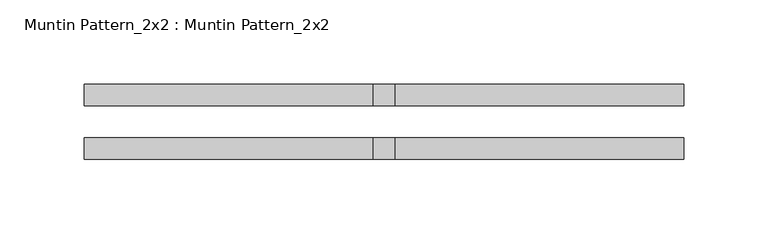
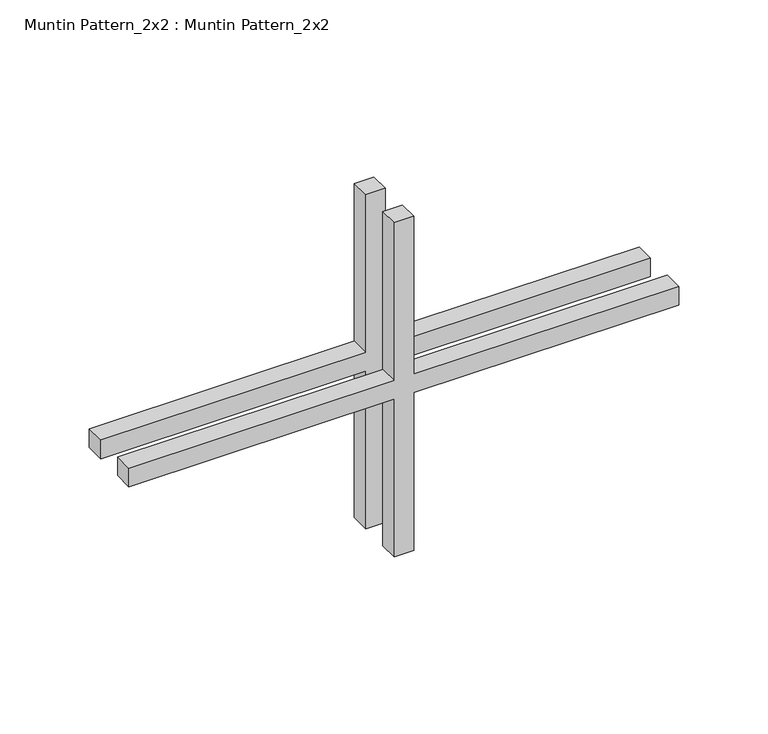
"""IFC4 building model written with IfcOpenShell, lengths in millimetres: proxy geometry, Muntin Pattern_2x2 : Muntin Pattern_2x2."""

from ifc_helpers import new_model, si_unit, frame, origin, place, context, project, spatial, polyline, outline, extrude, source, transform, mapped, element, save


def muntin_pattern_2x2_muntin_pattern_2x2_bb7dbb97(model_context):
    return source(origin(), model_context, "Body", "SweptSolid", [
        extrude(outline(polyline([(120.65, -6.35), (120.65, -177.8), (107.95, -177.8), (107.95, -6.35), (0.0, -6.35), (0.0, 6.35), (107.95, 6.35), (107.95, 177.8), (120.65, 177.8), (120.65, 6.35), (228.6, 6.35), (228.6, -6.35), (120.65, -6.35)])), frame((0.0, -22.225, 0.0), z_axis=(0.0, 1.0, 0.0), x_axis=(0.0, 0.0, 1.0)), (0.0, 0.0, 1.0), 12.7),
        extrude(outline(polyline([(120.65, -6.35), (120.65, -177.8), (107.95, -177.8), (107.95, -6.35), (0.0, -6.35), (0.0, 6.35), (107.95, 6.35), (107.95, 177.8), (120.65, 177.8), (120.65, 6.35), (228.6, 6.35), (228.6, -6.35), (120.65, -6.35)])), frame((0.0, 9.525, 0.0), z_axis=(0.0, 1.0, 0.0), x_axis=(0.0, 0.0, 1.0)), (0.0, 0.0, 1.0), 12.7),
    ])


if __name__ == "__main__":
    model = new_model("IFC4")
    model_context = context("Model", 3, world=origin())
    ifc_project = project(units=[si_unit("LENGTHUNIT", "METRE", prefix="MILLI")], contexts=[model_context])
    site = spatial("IfcSite", under=ifc_project)
    building = spatial("IfcBuilding", under=site)
    placement = place(None, origin())
    muntin_pattern_2x2_muntin_pattern_2x2_shape = muntin_pattern_2x2_muntin_pattern_2x2_bb7dbb97(model_context)
    element("IfcBuildingElementProxy", 1, Name="Muntin Pattern_2x2 : Muntin Pattern_2x2", ObjectType="Muntin Pattern_2x2 : Muntin Pattern_2x2", at=placement, inside=building, context=model_context, shape_type="MappedRepresentation", body=[
        mapped(muntin_pattern_2x2_muntin_pattern_2x2_shape, transform((0.0, 0.0, 0.0), x_axis=(1.0, 0.0, 0.0), y_axis=(0.0, 1.0, 0.0), z_axis=(0.0, 0.0, 1.0))),
    ])
    save(model, "model.ifc")

# Revit data of these elements
# Type "Muntin Pattern_2x2 : Muntin Pattern_2x2"
#   Width [instance default] = 4' - 0"
#   Thickness = 0' - 0 1/2"
#   Height [instance default] = 4' - 0"
#   Distance = 0' - 0 3/4"
#   Interior Material [instance default] = none
#   Exterior Material [instance default] = none
#   Default Elevation = 0
# Element 1 (IfcBuildingElementProxy, "Muntin Pattern_2x2 : Muntin Pattern_2x2")
#   Width = 1' - 2"
#   Height = 0' - 9"
#   Interior Material = Wood - Stained
#   Exterior Material = Clad - White
#   Materials on its faces: "Clad - White", "Wood - Stained"
# Materials
#   "Clad - White": class "Wood", colour RGB 242 242 238, transparency 0, Cost = 0
#   "Wood - Stained": class "Wood", colour RGB 224 178 126, transparency 0, Cost = 0
